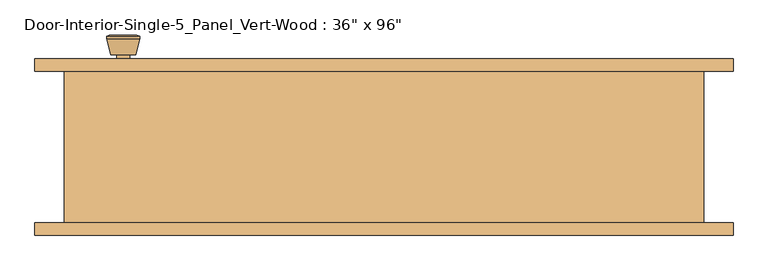
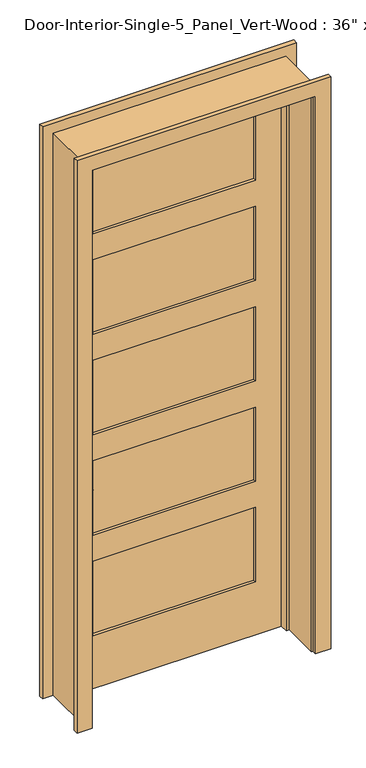
"""IFC4 building model written with IfcOpenShell, lengths in millimetres: door geometry."""

from ifc_helpers import new_model, si_unit, point, frame, frame_2d, origin, place, context, project, spatial, polyline, circle_curve, trimmed, segment, composite_curve, outline, extrude, faceted_brep, source, transform, mapped, element, save
from ifc_brep_helpers import plane_surface, cylinder_surface, revolved_surface, advanced_brep


def door_d793c26e(model_context):
    return source(origin(), model_context, "Body", "SolidModel", [
        advanced_brep(
        [(-393.7, 70.2, 914.4), (-383.7, 70.2, 914.4), (-403.7, 70.2, 914.4), (-373.2241324, 21.2, 914.4), (-393.7, 21.2, 914.4), (-414.1758676, 21.2, 914.4), (-368.7, 23.0278681, 914.4), (-418.7, 23.0278681, 914.4), (-368.7, 26.4915463, 914.4), (-418.7, 26.4915463, 914.4), (-375.063764, 51.2, 914.4), (-412.336236, 51.2, 914.4), (-383.7, 51.2, 914.4), (-403.7, 51.2, 914.4)],
        [
            (0, 1),
            (1, 2, circle_curve(frame((-393.7, 70.2, 914.4), z_axis=(0.0, 1.0, 0.0), x_axis=(-1.0, 0.0, 0.0)), 10.0)),
            (2, 0),
            (2, 1, circle_curve(frame((-393.7, 70.2, 914.4), z_axis=(0.0, 1.0, 0.0), x_axis=(-1.0, 0.0, 0.0)), 10.0)),
            (3, 4),
            (4, 5),
            (5, 3, circle_curve(frame((-393.7, 21.2, 914.4), z_axis=(0.0, -1.0, 0.0), x_axis=(-1.0, 0.0, 0.0)), 20.4758676)),
            (3, 5, circle_curve(frame((-393.7, 21.2, 914.4), z_axis=(0.0, -1.0, 0.0), x_axis=(-1.0, 0.0, 0.0)), 20.4758676)),
            (6, 3),
            (5, 7),
            (7, 6, circle_curve(frame((-393.7, 23.0278681, 914.4), z_axis=(0.0, -1.0, 0.0), x_axis=(-1.0, 0.0, 0.0)), 25.0)),
            (6, 7, circle_curve(frame((-393.7, 23.0278681, 914.4), z_axis=(0.0, -1.0, 0.0), x_axis=(-1.0, 0.0, 0.0)), 25.0)),
            (8, 6),
            (7, 9),
            (9, 8, circle_curve(frame((-393.7, 26.4915463, 914.4), z_axis=(0.0, -1.0, 0.0), x_axis=(-1.0, 0.0, 0.0)), 25.0)),
            (8, 9, circle_curve(frame((-393.7, 26.4915463, 914.4), z_axis=(0.0, -1.0, 0.0), x_axis=(-1.0, 0.0, 0.0)), 25.0)),
            (10, 8),
            (9, 11),
            (11, 10, circle_curve(frame((-393.7, 51.2, 914.4), z_axis=(0.0, -1.0, 0.0), x_axis=(-1.0, 0.0, 0.0)), 18.636236)),
            (10, 11, circle_curve(frame((-393.7, 51.2, 914.4), z_axis=(0.0, -1.0, 0.0), x_axis=(-1.0, 0.0, 0.0)), 18.636236)),
            (12, 10),
            (11, 13),
            (13, 12, circle_curve(frame((-393.7, 51.2, 914.4), z_axis=(0.0, -1.0, 0.0), x_axis=(-1.0, 0.0, 0.0)), 10.0)),
            (12, 13, circle_curve(frame((-393.7, 51.2, 914.4), z_axis=(0.0, -1.0, 0.0), x_axis=(-1.0, 0.0, 0.0)), 10.0)),
            (1, 12),
            (13, 2),
        ],
        [
            plane_surface(frame((-393.7, 70.2, 914.4), z_axis=(0.0, 1.0, 0.0), x_axis=(-1.0, 0.0, 0.0))),
            plane_surface(frame((-393.7, 21.2, 914.4), z_axis=(0.0, -1.0, 0.0), x_axis=(-1.0, 0.0, 0.0))),
            revolved_surface(polyline([(-414.1758676, 21.2, 914.4), (-418.7, 23.0278681, 914.4)]), (-393.7, 70.2, 914.4), (0.0, 1.0, 0.0)),
            cylinder_surface(frame((-393.7, 70.2, 914.4), z_axis=(0.0, 1.0, 0.0), x_axis=(-1.0, 0.0, 0.0)), 25.0),
            revolved_surface(polyline([(-418.7, 26.4915463, 914.4), (-412.336236, 51.2, 914.4)]), (-393.7, 70.2, 914.4), (0.0, 1.0, 0.0)),
            plane_surface(frame((-393.7, 51.2, 914.4), z_axis=(0.0, 1.0, 0.0), x_axis=(-1.0, 0.0, 0.0))),
            cylinder_surface(frame((-393.7, 70.2, 914.4), z_axis=(0.0, 1.0, 0.0), x_axis=(-1.0, 0.0, 0.0)), 10.0),
        ],
        [
            (0, [[1, 2, 3]]),
            (0, [[-3, 4, -1]]),
            (1, [[5, 6, 7]]),
            (1, [[-6, -5, 8]]),
            (2, [[9, -7, 10, 11]]),
            (2, [[-10, -8, -9, 12]]),
            (3, [[13, -11, 14, 15]]),
            (3, [[-14, -12, -13, 16]]),
            (4, [[17, -15, 18, 19]]),
            (4, [[-18, -16, -17, 20]]),
            (5, [[21, -19, 22, 23]]),
            (5, [[-22, -20, -21, 24]]),
            (6, [[25, -23, 26, -2]]),
            (6, [[-26, -24, -25, -4]]),
        ],
    ),
        extrude(outline(composite_curve([segment(trimmed(circle_curve(frame_2d((914.4, -393.7)), 30.0), [point((914.4, -423.7))], [point((914.4, -363.7))], False, "CARTESIAN"), True, "CONTINUOUS"), segment(trimmed(circle_curve(frame_2d((914.4, -393.7)), 30.0), [point((914.4, -363.7))], [point((914.4, -423.7))], False, "CARTESIAN"), True, "CONTINUOUS")], self_intersect=False)), frame((0.0, 70.2, 0.0), z_axis=(0.0, 1.0, 0.0), x_axis=(0.0, 0.0, 1.0)), (0.0, 0.0, 1.0), 6.0),
        advanced_brep(
        [(-393.7, 117.125, 914.4), (-403.7, 117.125, 914.4), (-383.7, 117.125, 914.4), (-373.2241324, 166.125, 914.4), (-414.1758676, 166.125, 914.4), (-393.7, 166.125, 914.4), (-368.7, 164.2971319, 914.4), (-418.7, 164.2971319, 914.4), (-368.7, 160.8334537, 914.4), (-418.7, 160.8334537, 914.4), (-375.063764, 136.125, 914.4), (-412.336236, 136.125, 914.4), (-383.7, 136.125, 914.4), (-403.7, 136.125, 914.4)],
        [
            (0, 1),
            (1, 2, circle_curve(frame((-393.7, 117.125, 914.4), z_axis=(0.0, -1.0, 0.0), x_axis=(-1.0, 0.0, 0.0)), 10.0)),
            (2, 0),
            (2, 1, circle_curve(frame((-393.7, 117.125, 914.4), z_axis=(0.0, -1.0, 0.0), x_axis=(-1.0, 0.0, 0.0)), 10.0)),
            (3, 4, circle_curve(frame((-393.7, 166.125, 914.4), z_axis=(0.0, 1.0, 0.0), x_axis=(-1.0, 0.0, 0.0)), 20.4758676)),
            (4, 5),
            (5, 3),
            (4, 3, circle_curve(frame((-393.7, 166.125, 914.4), z_axis=(0.0, 1.0, 0.0), x_axis=(-1.0, 0.0, 0.0)), 20.4758676)),
            (6, 7, circle_curve(frame((-393.7, 164.2971319, 914.4), z_axis=(0.0, 1.0, 0.0), x_axis=(-1.0, 0.0, 0.0)), 25.0)),
            (7, 4),
            (3, 6),
            (7, 6, circle_curve(frame((-393.7, 164.2971319, 914.4), z_axis=(0.0, 1.0, 0.0), x_axis=(-1.0, 0.0, 0.0)), 25.0)),
            (8, 9, circle_curve(frame((-393.7, 160.8334537, 914.4), z_axis=(0.0, 1.0, 0.0), x_axis=(-1.0, 0.0, 0.0)), 25.0)),
            (9, 7),
            (6, 8),
            (9, 8, circle_curve(frame((-393.7, 160.8334537, 914.4), z_axis=(0.0, 1.0, 0.0), x_axis=(-1.0, 0.0, 0.0)), 25.0)),
            (10, 11, circle_curve(frame((-393.7, 136.125, 914.4), z_axis=(0.0, 1.0, 0.0), x_axis=(-1.0, 0.0, 0.0)), 18.636236)),
            (11, 9),
            (8, 10),
            (11, 10, circle_curve(frame((-393.7, 136.125, 914.4), z_axis=(0.0, 1.0, 0.0), x_axis=(-1.0, 0.0, 0.0)), 18.636236)),
            (12, 13, circle_curve(frame((-393.7, 136.125, 914.4), z_axis=(0.0, 1.0, 0.0), x_axis=(-1.0, 0.0, 0.0)), 10.0)),
            (13, 11),
            (10, 12),
            (13, 12, circle_curve(frame((-393.7, 136.125, 914.4), z_axis=(0.0, 1.0, 0.0), x_axis=(-1.0, 0.0, 0.0)), 10.0)),
            (1, 13),
            (12, 2),
        ],
        [
            plane_surface(frame((-393.7, 117.125, 914.4), z_axis=(0.0, -1.0, 0.0), x_axis=(-1.0, 0.0, 0.0))),
            plane_surface(frame((-393.7, 166.125, 914.4), z_axis=(0.0, 1.0, 0.0), x_axis=(-1.0, 0.0, 0.0))),
            revolved_surface(polyline([(-414.1758676, 166.125, 914.4), (-418.7, 164.2971319, 914.4)]), (-393.7, 117.125, 914.4), (0.0, -1.0, 0.0)),
            cylinder_surface(frame((-393.7, 117.125, 914.4), z_axis=(0.0, -1.0, 0.0), x_axis=(-1.0, 0.0, 0.0)), 25.0),
            revolved_surface(polyline([(-418.7, 160.8334537, 914.4), (-412.336236, 136.125, 914.4)]), (-393.7, 117.125, 914.4), (0.0, -1.0, 0.0)),
            plane_surface(frame((-393.7, 136.125, 914.4), z_axis=(0.0, -1.0, 0.0), x_axis=(-1.0, 0.0, 0.0))),
            cylinder_surface(frame((-393.7, 117.125, 914.4), z_axis=(0.0, -1.0, 0.0), x_axis=(-1.0, 0.0, 0.0)), 10.0),
        ],
        [
            (0, [[1, 2, 3]]),
            (0, [[-3, 4, -1]]),
            (1, [[5, 6, 7]]),
            (1, [[8, -7, -6]]),
            (2, [[9, 10, -5, 11]]),
            (2, [[12, -11, -8, -10]]),
            (3, [[13, 14, -9, 15]]),
            (3, [[16, -15, -12, -14]]),
            (4, [[17, 18, -13, 19]]),
            (4, [[20, -19, -16, -18]]),
            (5, [[21, 22, -17, 23]]),
            (5, [[24, -23, -20, -22]]),
            (6, [[-2, 25, -21, 26]]),
            (6, [[-4, -26, -24, -25]]),
        ],
    ),
        extrude(outline(composite_curve([segment(trimmed(circle_curve(frame_2d((914.4, -393.7)), 30.0), [point((914.4, -423.7))], [point((914.4, -363.7))], False, "CARTESIAN"), True, "CONTINUOUS"), segment(trimmed(circle_curve(frame_2d((914.4, -393.7)), 30.0), [point((914.4, -363.7))], [point((914.4, -423.7))], False, "CARTESIAN"), True, "CONTINUOUS")], self_intersect=False)), frame((0.0, 111.125, 0.0), z_axis=(0.0, 1.0, 0.0), x_axis=(0.0, 0.0, 1.0)), (0.0, 0.0, 1.0), 6.0),
        faceted_brep([(482.6, 111.125, 0.0), (482.6, -117.475, 0.0), (457.2, -117.475, 0.0), (457.2, 41.275, 0.0), (444.5, 41.275, 0.0), (444.5, 76.2, 0.0), (457.2, 76.2, 0.0), (457.2, 111.125, 0.0), (482.6, 111.125, 2463.8), (482.6, -117.475, 2463.8), (-482.6, -117.475, 2463.8), (-482.6, -117.475, 0.0), (-457.2, -117.475, 0.0), (-457.2, -117.475, 2438.4), (457.2, -117.475, 2438.4), (457.2, 41.275, 2438.4), (-457.2, 41.275, 2438.4), (-457.2, 41.275, 0.0), (-444.5, 41.275, 0.0), (-444.5, 41.275, 2425.7), (444.5, 41.275, 2425.7), (444.5, 76.2, 2425.7), (-444.5, 76.2, 2425.7), (-444.5, 76.2, 0.0), (-457.2, 76.2, 0.0), (-457.2, 76.2, 2438.4), (457.2, 76.2, 2438.4), (457.2, 111.125, 2438.4), (-457.2, 111.125, 2438.4), (-457.2, 111.125, 0.0), (-482.6, 111.125, 0.0), (-482.6, 111.125, 2463.8)], [[[0, 1, 2, 3, 4, 5, 6, 7]], [[1, 0, 8, 9]], [[2, 1, 9, 10, 11, 12, 13, 14]], [[3, 2, 14, 15]], [[4, 3, 15, 16, 17, 18, 19, 20]], [[5, 4, 20, 21]], [[6, 5, 21, 22, 23, 24, 25, 26]], [[7, 6, 26, 27]], [[0, 7, 27, 28, 29, 30, 31, 8]], [[9, 8, 31, 10]], [[15, 14, 13, 16]], [[21, 20, 19, 22]], [[27, 26, 25, 28]], [[30, 29, 24, 23, 18, 17, 12, 11]], [[10, 31, 30, 11]], [[16, 13, 12, 17]], [[22, 19, 18, 23]], [[28, 25, 24, 29]]]),
        extrude(outline(polyline([(2438.4, -457.2), (0.0, -457.2), (0.0, 457.2), (2438.4, 457.2), (2438.4, -457.2)]), holes=[polyline([(2319.3375, -336.55), (2319.3375, 336.55), (1993.265, 336.55), (1993.265, -336.55), (2319.3375, -336.55)]), polyline([(557.8475, -336.55), (557.8475, 336.55), (231.775, 336.55), (231.775, -336.55), (557.8475, -336.55)]), polyline([(1438.5925, -336.55), (1438.5925, 336.55), (1112.52, 336.55), (1112.52, -336.55), (1438.5925, -336.55)]), polyline([(1878.965, -336.55), (1878.965, 336.55), (1552.8925, 336.55), (1552.8925, -336.55), (1878.965, -336.55)]), polyline([(998.22, -336.55), (998.22, 336.55), (672.1475, 336.55), (672.1475, -336.55), (998.22, -336.55)])]), frame((0.0, 76.2, 0.0), z_axis=(0.0, 1.0, 0.0), x_axis=(0.0, 0.0, 1.0)), (0.0, 0.0, 1.0), 34.925),
        extrude(outline(polyline([(336.55, 87.8416667), (-336.55, 87.8416667), (-336.55, 99.4833333), (336.55, 99.4833333), (336.55, 87.8416667)])), frame((0.0, 0.0, 1993.265), z_axis=(0.0, 0.0, 1.0), x_axis=(1.0, 0.0, 0.0)), (0.0, 0.0, 1.0), 326.0725),
        extrude(outline(polyline([(336.55, 87.8416667), (-336.55, 87.8416667), (-336.55, 99.4833333), (336.55, 99.4833333), (336.55, 87.8416667)])), frame((0.0, 0.0, 1552.8925), z_axis=(0.0, 0.0, 1.0), x_axis=(1.0, 0.0, 0.0)), (0.0, 0.0, 1.0), 326.0725),
        extrude(outline(polyline([(336.55, 87.8416667), (-336.55, 87.8416667), (-336.55, 99.4833333), (336.55, 99.4833333), (336.55, 87.8416667)])), frame((0.0, 0.0, 672.1475), z_axis=(0.0, 0.0, 1.0), x_axis=(1.0, 0.0, 0.0)), (0.0, 0.0, 1.0), 326.0725),
        extrude(outline(polyline([(336.55, 87.8416667), (-336.55, 87.8416667), (-336.55, 99.4833333), (336.55, 99.4833333), (336.55, 87.8416667)])), frame((0.0, 0.0, 231.775), z_axis=(0.0, 0.0, 1.0), x_axis=(1.0, 0.0, 0.0)), (0.0, 0.0, 1.0), 326.0725),
        extrude(outline(polyline([(336.55, 87.8416667), (-336.55, 87.8416667), (-336.55, 99.4833333), (336.55, 99.4833333), (336.55, 87.8416667)])), frame((0.0, 0.0, 1112.52), z_axis=(0.0, 0.0, 1.0), x_axis=(1.0, 0.0, 0.0)), (0.0, 0.0, 1.0), 326.0725),
        extrude(outline(polyline([(0.0, 463.55), (0.0, 527.05), (2508.25, 527.05), (2508.25, -527.05), (0.0, -527.05), (0.0, -463.55), (2444.75, -463.55), (2444.75, 463.55), (0.0, 463.55)])), frame((0.0, 111.125, 0.0), z_axis=(0.0, 1.0, 0.0), x_axis=(0.0, 0.0, 1.0)), (0.0, 0.0, 1.0), 19.05),
        extrude(outline(polyline([(0.0, 463.55), (0.0, 527.05), (2508.25, 527.05), (2508.25, -527.05), (0.0, -527.05), (0.0, -463.55), (2444.75, -463.55), (2444.75, 463.55), (0.0, 463.55)])), frame((0.0, -136.525, 0.0), z_axis=(0.0, 1.0, 0.0), x_axis=(0.0, 0.0, 1.0)), (0.0, 0.0, 1.0), 19.05),
    ])


if __name__ == "__main__":
    model = new_model("IFC4")
    model_context = context("Model", 3, world=origin())
    ifc_project = project(units=[si_unit("LENGTHUNIT", "METRE", prefix="MILLI")], contexts=[model_context])
    site = spatial("IfcSite", under=ifc_project)
    building = spatial("IfcBuilding", under=site)
    placement = place(None, origin())
    door_shape = door_d793c26e(model_context)
    element("IfcDoor", 1, ObjectType="Door-Interior-Single-5_Panel_Vert-Wood : 36\" x 96\"", at=placement, inside=building, context=model_context, shape_type="MappedRepresentation", body=[
        mapped(door_shape, transform((0.0, 0.0, 0.0), x_axis=(1.0, 0.0, 0.0), y_axis=(0.0, 1.0, 0.0), z_axis=(0.0, 0.0, 1.0))),
    ])
    save(model, "model.ifc")

# Revit data of these elements
# Type "Door-Interior-Single-5_Panel_Vert-Wood : 36\" x 96\""
#   Type Mark = "8"
#   Assembly Code = "C1020300"
#   Analytic Construction = "Wooden"
#   Top Rail = 0' - 4 11/16"
#   Thickness = 0' - 1 3/8"
#   Thermal Resistance (R) = 2.5876 (h·ft²·°F)/BTU
#   Swing Angle [instance default] = 90.00°
#   Stiles = 0' - 4 3/4"
#   Rough Width = 3' - 2"
#   Rough Height = 8' - 1"
#   Intermediate Rail = 0' - 4 1/2"
#   Height = 8' - 0"
#   Width = 3' - 0"
#   Heat Transfer Coefficient (U) = 0.3865 BTU/(h·ft²·°F)
#   Bottom Rail = 0' - 9 1/8"
#   Trim Material = Cherry
#   Panel Material = Cherry
#   Frame Material = Cherry
#   Door Handle Material = Aluminum
#   Visual Light Transmittance = 0
#   Solar Heat Gain Coefficient = 0
#   Wall Closure = (empty or 0)
#   Function = (empty or 0)
# Element 1 (IfcDoor, "Door-Interior-Single-5_Panel_Vert-Wood : 36\" x 96\"")
#   Materials on its faces: "Cherry", "Aluminum"
# Materials
#   "Cherry": class "Wood", colour RGB 226 177 128, transparency 0, Description = "Prunus Serotina", Cost = 0
#   "Aluminum": class "Metal", colour RGB 247 247 247, transparency 0, Description = "Aluminum 6061", Cost = 0
